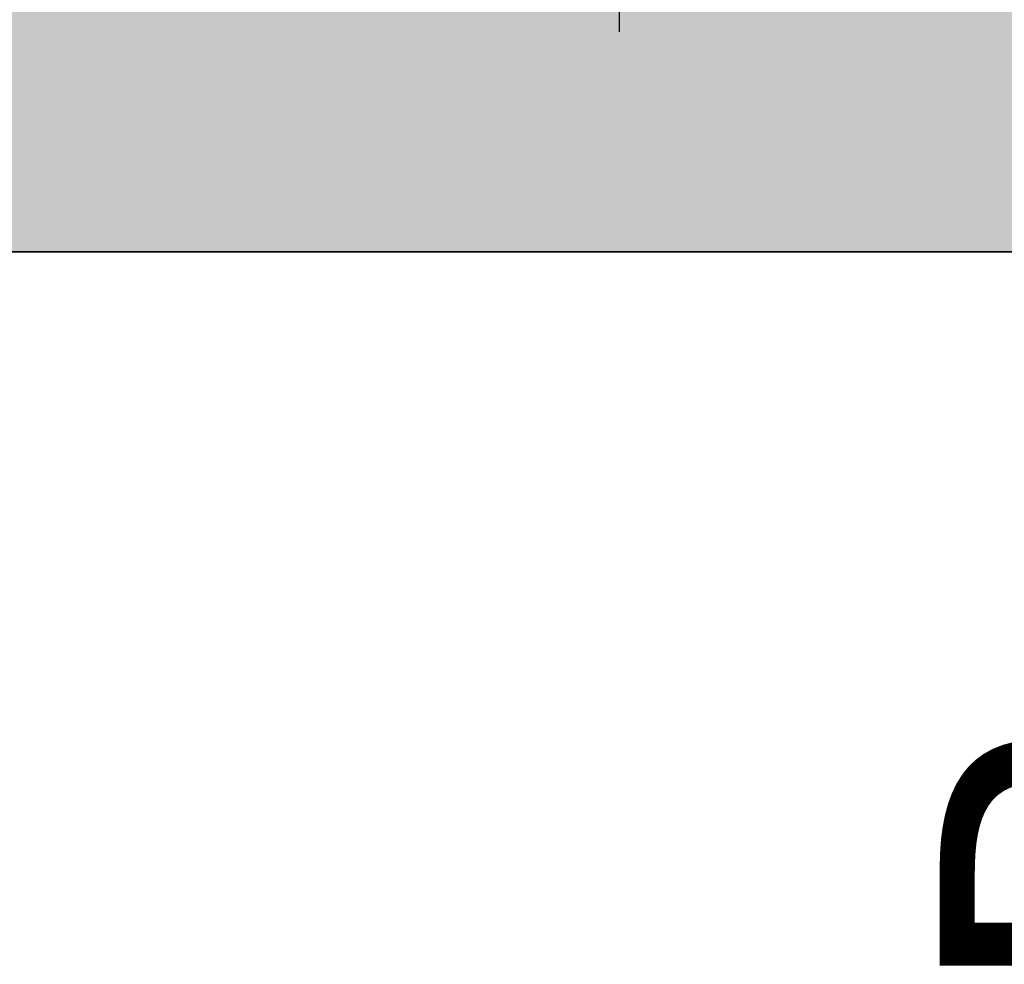
# Model space of a CAD drawing. Units: inches. Extents: x 2083 to 3317, y 1141 to 2115.
# Tile 123 of 256: x 3068 to 3102, y 1238 to 1271. Entities that reach past the tile are written whole.
import ezdxf

# ---------------------------------------------------------------- set-up
doc = ezdxf.new("R2010")
doc.units = ezdxf.units.IN
doc.layers.add('A-ANNO-DIMS', color=2, linetype='Continuous', lineweight=18)
doc.layers.add('A-WALL', color=7, linetype='Continuous', lineweight=35)
doc.layers.add('A-WALL-PATT', color=251, linetype='Continuous', lineweight=13, true_color=0x636466)
doc.styles.get("Standard").update_dxf_attribs({"font": 'arial.ttf'})
doc.dimstyles.new('ISO-25', dxfattribs={"dimtxt": 12, "dimasz": 12, "dimexe": 1.25, "dimexo": 0.625, "dimtad": 1, "dimlunit": 3, "dimtxsty": 'Standard', "dimcen": 2.5, "dimadec": 0, "dimazin": 0, "dimtfac": 1, "dimtmove": 0, "dimatfit": 3, "dimfxl": 1, "dimarcsym": 0})

# ---------------------------------------------------------------- blocks, each defined once
blk = doc.blocks.new('*D10')
at = {"layer": 'A-ANNO-DIMS', "color": 0, "lineweight": -2, "transparency": 16777216}
for p, q in [((2862.96, 1262.636), (2862.96, 1201.384)), ((3126.96, 1262.636), (3126.96, 1201.384)), ((2874.96, 1202.634), (3114.96, 1202.634))]:
    blk.add_line(p, q, dxfattribs=at)
at = {"layer": 'A-ANNO-DIMS', "color": 0, "transparency": 16777216}
for points in [[(2874.96, 1204.634), (2874.96, 1200.634), (2862.96, 1202.634)], [(3114.96, 1204.634), (3114.96, 1200.634), (3126.96, 1202.634)]]:
    blk.add_solid(points, dxfattribs=at)
at = {"layer": 'Defpoints', "color": 0, "transparency": 16777216}
for p in [(2862.96, 1263.261), (3126.96, 1263.261), (3126.96, 1202.634)]:
    blk.add_point(p, dxfattribs=at)
at = {"layer": 'A-ANNO-DIMS', "color": 0, "transparency": 16777216, "insert": (2994.96, 1209.284), "char_height": 12, "attachment_point": 5}
blk.add_mtext("22'", dxfattribs=at)
blk = doc.blocks.new('*D26')
at = {"layer": 'A-ANNO-DIMS', "color": 0, "lineweight": -2, "transparency": 16777216}
for p, q in [((3088.986, 1274.915), (3088.986, 1270.952)), ((3111.24, 1274.915), (3111.24, 1270.952)), ((3076.986, 1272.202), (2840.262, 1272.202)), ((3111.24, 1272.202), (3088.986, 1272.202)), ((3123.24, 1272.202), (3135.24, 1272.202))]:
    blk.add_line(p, q, dxfattribs=at)
at = {"layer": 'A-ANNO-DIMS', "color": 0, "transparency": 16777216}
for points in [[(3076.986, 1274.202), (3076.986, 1270.202), (3088.986, 1272.202)], [(3123.24, 1274.202), (3123.24, 1270.202), (3111.24, 1272.202)]]:
    blk.add_solid(points, dxfattribs=at)
at = {"layer": 'Defpoints', "color": 0, "transparency": 16777216}
for p in [(3088.986, 1275.54), (3111.24, 1275.54), (3088.986, 1272.202)]:
    blk.add_point(p, dxfattribs=at)
at = {"layer": 'A-ANNO-DIMS', "color": 0, "transparency": 16777216, "insert": (2952.624, 1279.032), "char_height": 12, "attachment_point": 5}
blk.add_mtext('NIGHTSTAND 1\'-10 1/2" TYP.', dxfattribs=at)
blk = doc.blocks.new('*D27')
at = {"layer": 'A-ANNO-DIMS', "color": 0, "lineweight": -2, "transparency": 16777216}
for p, q in [((3114.578, 1309.794), (3114.578, 1321.794)), ((3111.865, 1297.794), (3115.828, 1297.794)), ((3114.578, 1297.794), (3114.578, 1275.54)), ((3111.865, 1275.54), (3115.828, 1275.54)), ((3114.578, 1263.54), (3114.578, 1140.989))]:
    blk.add_line(p, q, dxfattribs=at)
at = {"layer": 'A-ANNO-DIMS', "color": 0, "transparency": 16777216}
for points in [[(3112.578, 1309.794), (3116.578, 1309.794), (3114.578, 1297.794)], [(3112.578, 1263.54), (3116.578, 1263.54), (3114.578, 1275.54)]]:
    blk.add_solid(points, dxfattribs=at)
at = {"layer": 'Defpoints', "color": 0, "transparency": 16777216}
for p in [(3111.24, 1297.794), (3111.24, 1275.54), (3114.578, 1275.54)]:
    blk.add_point(p, dxfattribs=at)
at = {"layer": 'A-ANNO-DIMS', "color": 0, "transparency": 16777216, "insert": (3107.749, 1196.264), "char_height": 12, "attachment_point": 5, "rotation": 90}
blk.add_mtext('1\'-10 1/2" TYP.', dxfattribs=at)
blk = doc.blocks.new('*D34')
at = {"layer": 'A-ANNO-DIMS', "color": 0, "lineweight": -2, "transparency": 16777216}
for p, q in [((2226.96, 1262.636), (2226.96, 1209.661)), ((3126.96, 1262.636), (3126.96, 1209.661)), ((2238.96, 1210.911), (3114.96, 1210.911))]:
    blk.add_line(p, q, dxfattribs=at)
at = {"layer": 'A-ANNO-DIMS', "color": 0, "transparency": 16777216}
for points in [[(2238.96, 1212.911), (2238.96, 1208.911), (2226.96, 1210.911)], [(3114.96, 1212.911), (3114.96, 1208.911), (3126.96, 1210.911)]]:
    blk.add_solid(points, dxfattribs=at)
at = {"layer": 'Defpoints', "color": 0, "transparency": 16777216}
for p in [(2226.96, 1263.261), (3126.96, 1263.261), (3126.96, 1210.911)]:
    blk.add_point(p, dxfattribs=at)
at = {"layer": 'A-ANNO-DIMS', "color": 0, "transparency": 16777216, "insert": (2676.96, 1217.663), "char_height": 12, "attachment_point": 5}
blk.add_mtext('75\'-0"', dxfattribs=at)

msp = doc.modelspace()

# ---------------------------------------------------------------- hatches: boundary and pattern name
at = {"layer": 'A-WALL-PATT'}
h = msp.add_hatch(color=256, dxfattribs=at)
h.dxf.hatch_style = 1
h.paths.add_polyline_path([(3126.96, 2020.761), (2748.96, 2020.761), (2604.96, 2020.761), (2226.96, 2020.761), (2226.96, 1702.761), (2466.96, 1702.761), (2466.96, 1582.761), (2418.96, 1582.761), (2418.96, 1477.761), (2226.96, 1477.761), (2226.96, 1263.261), (2544.96, 1263.261), (2544.96, 1411.761), (2604.96, 1411.761), (2685.96, 1411.761), (2685.96, 1420.761), (2604.96, 1420.761), (2604.96, 1573.761), (2604.96, 1702.761), (2604.96, 2011.761), (2748.96, 2011.761), (2748.96, 1702.761), (2862.96, 1702.761), (2862.96, 1621.761), (2871.96, 1621.761), (2871.96, 1702.761), (2883.96, 1702.761), (2883.96, 1706.939, -0.026459), (2883.96, 1711.761), (2757.96, 1711.761), (2757.96, 1807.761), (2787.96, 1807.761), (2787.96, 1812.261), (2757.96, 1812.261), (2757.96, 2011.761), (2877.96, 2011.761), (2877.96, 1812.261), (2847.96, 1812.261), (2847.96, 1807.761), (2889.836, 1807.761), (2889.836, 1812.261), (2882.46, 1812.261), (2882.46, 2011.761), (3117.96, 2011.761), (3117.96, 1812.261), (2937.836, 1812.261), (2937.836, 1807.761), (2995.71, 1807.761), (2995.71, 1796.118), (3000.21, 1796.118), (3000.21, 1807.761), (3117.96, 1807.761), (3117.96, 1711.761), (3000.21, 1711.761), (3000.21, 1760.118), (2998.573, 1760.118, -0.020711), (2995.71, 1760.118), (2995.71, 1711.761), (2931.96, 1711.761), (2931.96, 1702.761), (3126.96, 1702.761)])
h.paths.add_polyline_path([(2471.46, 2011.761), (2471.46, 1810.011), (2462.717, 1810.011), (2462.717, 1805.511), (2505.96, 1805.511), (2505.96, 1810.011), (2475.96, 1810.011), (2475.96, 2011.761), (2595.96, 2011.761), (2595.96, 1810.011), (2565.96, 1810.011), (2565.96, 1805.511), (2595.96, 1805.511), (2595.96, 1711.761), (2235.96, 1711.761), (2235.96, 1805.511), (2353.71, 1805.511), (2353.71, 1796.054), (2358.21, 1796.054), (2358.21, 1805.511), (2414.717, 1805.511), (2414.717, 1810.011), (2235.96, 1810.011), (2235.96, 2011.761)], flags=16)
h.paths.add_polyline_path([(2270.205, 1994.61), (2270.205, 1970.61), (2246.205, 1970.61), (2246.205, 1994.61)], flags=0)
edge = h.paths.add_edge_path(flags=0)
edge.add_ellipse((2332.027, 1899.798), major_axis=(-3.043, 3.043), ratio=0.168252, start_angle=-161.3322, end_angle=-156.3071, ccw=False)
edge.add_ellipse((2333.082, 1898.744), major_axis=(-1.055, 1.055), ratio=0.453532, start_angle=-123.371, end_angle=-94.1591)
edge = h.paths.add_edge_path(flags=0)
edge.add_ellipse((2332.027, 1968.876), major_axis=(3.043, 3.043), ratio=0.168252, start_angle=18.6678, end_angle=23.6929)
edge.add_spline(control_points=[(2332.926, 1970.691), (2332.227, 1970.336), (2330.894, 1969.659), (2328.413, 1970.932), (2327.204, 1967.749), (2324.71, 1969.956), (2322.533, 1967.012), (2320.013, 1971.296), (2317.68, 1968.158), (2316.041, 1967.102), (2315.427, 1966.81)], knot_values=[0, 0, 0, 0, 2.267059, 4.324559, 6.685584, 8.878641, 11.121502, 14.300359, 17.755284, 19.732645, 19.732645, 19.732645, 19.732645], degree=3, periodic=0)
edge.add_ellipse((2332.027, 1968.876), major_axis=(3.043, 3.043), ratio=0.168252, start_angle=18.6678, end_angle=23.6929, ccw=False)
edge.add_ellipse((2333.082, 1969.931), major_axis=(1.055, 1.055), ratio=0.453532, start_angle=56.629, end_angle=85.8409, ccw=False)
edge = h.paths.add_edge_path(flags=0)
edge.add_spline(control_points=[(2296.428, 1967.988), (2293.628, 1965.336), (2287.704, 1959.727), (2299.744, 1949.996), (2294.533, 1935.669), (2290.573, 1920.604), (2293.394, 1909.974), (2296.185, 1904.967)], knot_values=[0.099185, 0.099185, 0.099185, 0.099185, 0.345301, 0.619822, 0.982653, 1.386093, 1.810555, 1.810555, 1.810555, 1.810555], degree=3, periodic=0)
edge.add_spline(control_points=[(2296.185, 1904.967), (2297.384, 1902.619), (2298.001, 1901.949), (2298.553, 1901.468)], knot_values=[0.006246, 0.006246, 0.006246, 0.006246, 0.055476, 0.055476, 0.055476, 0.055476], degree=3, periodic=0)
edge.add_spline(control_points=[(2298.553, 1901.468), (2297.259, 1900.923), (2295.225, 1900.232), (2293.06, 1900.614), (2292.101, 1900.788), (2292.09, 1900.791)], knot_values=[0.312835, 0.312835, 0.312835, 0.312835, 0.40178, 0.474987, 0.475903, 0.475903, 0.475903, 0.475903], degree=3, periodic=0)
edge.add_arc((2292.794, 1904.664), 3.937, 215.4209, 259.6982, ccw=False)
edge.add_spline(control_points=[(2289.585, 1902.382), (2289.477, 1902.535), (2289.368, 1902.688), (2289.261, 1902.841)], knot_values=[0.102872, 0.102872, 0.102872, 0.102872, 0.116896, 0.116896, 0.116896, 0.116896], degree=3, periodic=0)
edge.add_spline(control_points=[(2289.261, 1902.841), (2288.687, 1902.55), (2287.64, 1902.02), (2285.881, 1901.874), (2283.853, 1901.504), (2281.72, 1899.711), (2278.467, 1899.493), (2276.157, 1901.883), (2272.259, 1899.804), (2267.778, 1901.843), (2262.244, 1900.184), (2257.415, 1901.782), (2254.318, 1900.726), (2253.178, 1900.337)], knot_values=[0, 0, 0, 0, 1.907977, 3.477176, 5.261074, 7.972851, 11.680248, 13.717921, 16.939592, 22.789562, 27.502503, 33.595215, 37.145618, 37.145618, 37.145618, 37.145618], degree=3, periodic=0)
edge.add_line((2253.178, 1900.337), (2250.244, 1902.841))
edge.add_line((2250.244, 1902.841), (2250.244, 1965.833))
edge.add_line((2250.244, 1965.833), (2253.178, 1968.337))
edge.add_spline(control_points=[(2253.178, 1968.337), (2254.318, 1967.948), (2257.415, 1966.892), (2262.244, 1968.49), (2267.778, 1966.831), (2271.527, 1968.537), (2273.876, 1967.828), (2274.207, 1967.728)], knot_values=[0, 0, 0, 0, 0.09018, 0.244935, 0.364644, 0.513233, 0.537855, 0.537855, 0.537855, 0.537855], degree=3, periodic=0)
edge.add_arc((2274.353, 1963.793), 3.937, 72.0511, 92.1279, ccw=False)
edge.add_arc((2281.297, 1985.23), 18.596, 252.0511, 288.5657)
edge.add_arc((2292.317, 1956.029), 12.646, 71.0268, 113.7782, ccw=False)
edge = h.paths.add_edge_path(flags=0)
edge.add_spline(control_points=[(2274.899, 1951.856), (2275.066, 1951.617), (2275.233, 1951.377), (2275.398, 1951.136)], knot_values=[1.409916, 1.409916, 1.409916, 1.409916, 1.43159, 1.43159, 1.43159, 1.43159], degree=3, periodic=0)
edge.add_spline(control_points=[(2275.398, 1951.136), (2275.792, 1950.562), (2276.179, 1949.984), (2276.546, 1949.397)], knot_values=[1.358238, 1.358238, 1.358238, 1.358238, 1.409916, 1.409916, 1.409916, 1.409916], degree=3, periodic=0)
edge.add_line((2276.546, 1949.397), (2277.437, 1947.862))
edge.add_spline(control_points=[(2277.437, 1947.862), (2276.304, 1945.673), (2274.64, 1942.427), (2274.632, 1938.094), (2272.799, 1930.852), (2274.356, 1943.897), (2275.948, 1947.923), (2276.546, 1949.397)], knot_values=[0.005632, 0.005632, 0.005632, 0.005632, 0.186014, 0.266002, 0.357087, 0.59639, 0.739732, 0.739732, 0.739732, 0.739732], degree=3, periodic=0)
edge.add_spline(control_points=[(2276.546, 1949.397), (2276.179, 1949.984), (2275.792, 1950.562), (2275.398, 1951.136)], knot_values=[1.358238, 1.358238, 1.358238, 1.358238, 1.409916, 1.409916, 1.409916, 1.409916], degree=3, periodic=0)
edge.add_spline(control_points=[(2275.398, 1951.136), (2274.943, 1950.08), (2274.208, 1948.025), (2273.935, 1944.851), (2272.469, 1937.627), (2273.466, 1945.696), (2274.701, 1951.059), (2274.899, 1951.856)], knot_values=[0.104364, 0.104364, 0.104364, 0.104364, 0.189636, 0.269624, 0.36071, 0.600013, 0.644622, 0.644622, 0.644622, 0.644622], degree=3, periodic=0)
h.paths.add_polyline_path([(2269.168, 1963.128, -0.357527), (2268.171, 1960.976, -0.092561), (2268.171, 1939.436, -0.357527), (2269.168, 1937.285, -0.357527), (2267.016, 1938.282, -0.164785), (2254.686, 1938.282, -0.357527), (2252.534, 1937.285, -0.357527), (2253.531, 1939.436, -0.092561), (2253.531, 1960.976, -0.357527), (2252.534, 1963.128, -0.357527), (2254.686, 1962.131, -0.164785), (2267.016, 1962.131, -0.357527)], flags=0)
h.paths.add_polyline_path([(2248.874, 1967.802), (2248.874, 1957.028), (2249.458, 1957.028), (2249.458, 1911.647), (2248.874, 1911.647), (2248.874, 1900.873), (2246.512, 1900.873, 0.197327), (2244.15, 1902.457), (2244.15, 1966.218, 0.197327), (2246.512, 1967.802)], flags=0)
h.paths.add_polyline_path([(2269.168, 1931.389, -0.357527), (2268.171, 1929.238, -0.092561), (2268.171, 1907.698, -0.357527), (2269.168, 1905.547, -0.357527), (2267.016, 1906.544, -0.164785), (2254.686, 1906.544, -0.357527), (2252.534, 1905.547, -0.357527), (2253.531, 1907.698, -0.092561), (2253.531, 1929.238, -0.357527), (2252.534, 1931.389, -0.357527), (2254.686, 1930.392, -0.164785), (2267.016, 1930.392, -0.357527)], flags=0)
edge = h.paths.add_edge_path(flags=0)
edge.add_spline(control_points=[(2276.197, 1906.724), (2276.168, 1909.029), (2276.114, 1913.372), (2270.598, 1924.925), (2273.905, 1919.013), (2275.922, 1916.262), (2275.475, 1912.402), (2277.258, 1910.381), (2276.696, 1908.225), (2276.646, 1906.813), (2276.618, 1906.008)], knot_values=[0, 0, 0, 0, 8.61026, 16.221274, 18.843057, 23.804898, 27.440828, 29.356102, 31.203478, 33.650687, 33.650687, 33.650687, 33.650687], degree=3, periodic=0)
edge.add_spline(control_points=[(2276.618, 1906.008), (2276.623, 1905.624), (2276.498, 1904.629), (2275.442, 1903.855), (2274.937, 1903.08), (2274.859, 1902.841)], knot_values=[0.156488, 0.156488, 0.156488, 0.156488, 0.184398, 0.231376, 0.250598, 0.250598, 0.250598, 0.250598], degree=3, periodic=0)
edge.add_line((2274.859, 1902.841), (2276.506, 1902.841))
edge.add_spline(control_points=[(2276.506, 1902.841), (2276.788, 1903.085), (2277.665, 1904.125), (2278.25, 1904.341), (2277.654, 1908.527), (2278.156, 1906.228), (2278.1, 1905.286), (2278.847, 1904.069), (2277.857, 1903.415), (2277.874, 1902.991), (2277.904, 1902.841)], knot_values=[0.059574, 0.059574, 0.059574, 0.059574, 0.080753, 0.103741, 0.16972, 0.176036, 0.207137, 0.240474, 0.262341, 0.27366, 0.27366, 0.27366, 0.27366], degree=3, periodic=0)
edge.add_line((2277.904, 1902.841), (2280.03, 1902.841))
edge.add_spline(control_points=[(2280.03, 1902.841), (2279.888, 1903.088), (2279.499, 1903.982), (2280.152, 1905.939), (2278.104, 1909.658), (2279.762, 1907.185), (2280.328, 1904.875), (2280.485, 1903.49), (2281.463, 1903.249), (2281.758, 1902.936), (2281.834, 1902.841)], knot_values=[0.013856, 0.013856, 0.013856, 0.013856, 0.034874, 0.088867, 0.107879, 0.126738, 0.158714, 0.193757, 0.217487, 0.226722, 0.226722, 0.226722, 0.226722], degree=3, periodic=0)
edge.add_spline(control_points=[(2281.834, 1902.841), (2281.788, 1902.827), (2281.647, 1902.783), (2281.396, 1902.859), (2281.088, 1902.985), (2280.721, 1903.061), (2280.333, 1903.026), (2280.125, 1902.899), (2280.03, 1902.841)], knot_values=[0, 0, 0, 0, 0.14413, 0.435517, 0.749276, 1.153046, 1.548371, 1.878348, 1.878348, 1.878348, 1.878348], degree=3, periodic=0)
edge.add_line((2280.03, 1902.841), (2277.904, 1902.841))
edge.add_spline(control_points=[(2277.904, 1902.841), (2277.893, 1902.796), (2277.865, 1902.68), (2277.607, 1902.687), (2277.274, 1902.801), (2276.838, 1902.62), (2276.584, 1902.789), (2276.506, 1902.841)], knot_values=[0, 0, 0, 0, 0.127189, 0.326199, 0.628009, 1.24357, 1.515331, 1.515331, 1.515331, 1.515331], degree=3, periodic=0)
edge.add_line((2276.506, 1902.841), (2274.859, 1902.841))
edge.add_spline(control_points=[(2274.859, 1902.841), (2274.814, 1902.899), (2274.725, 1903.013), (2274.493, 1903.119), (2274.244, 1902.961), (2273.937, 1903.185), (2273.614, 1902.983), (2273.408, 1902.883), (2273.322, 1902.841)], knot_values=[0, 0, 0, 0, 0.21843, 0.436957, 0.687977, 0.990379, 1.398396, 1.69185, 1.69185, 1.69185, 1.69185], degree=3, periodic=0)
edge.add_spline(control_points=[(2273.322, 1902.841), (2273.617, 1903.446), (2274.274, 1904.538), (2276.027, 1904.574), (2276.207, 1906.584), (2276.197, 1906.724)], knot_values=[0.012227, 0.012227, 0.012227, 0.012227, 0.059472, 0.106218, 0.134458, 0.134458, 0.134458, 0.134458], degree=3, periodic=0)
h.paths.add_polyline_path([(2270.776, 1897.79), (2270.776, 1873.79), (2246.776, 1873.79), (2246.776, 1897.79)], flags=0)
h.paths.add_polyline_path([(2353.71, 1760.005), (2353.71, 1760.054), (2358.21, 1760.054, -0.033729)], flags=0)
h.paths.add_polyline_path([(2321.819, 1737.529), (2341.995, 1737.529, -0.414214), (2343.203, 1736.321), (2343.203, 1721.021, -0.414214), (2341.995, 1719.813), (2321.819, 1719.813, -0.414214), (2320.611, 1721.021), (2320.611, 1736.321, -0.414214)], flags=0)
h.paths.add_polyline_path([(2324.235, 1736.321), (2339.579, 1736.321, -0.414214), (2341.995, 1733.905), (2341.995, 1725.45, -0.414214), (2339.579, 1723.034), (2333.681, 1723.034), (2333.845, 1722.045, -0.870646), (2335.425, 1721.826, -0.767327), (2333.923, 1721.423), (2331.291, 1721.423, -0.767327), (2329.788, 1721.826, -0.870646), (2331.368, 1722.045), (2331.533, 1723.034), (2324.235, 1723.034, -0.414214), (2321.819, 1725.45), (2321.819, 1733.905, -0.414214)], flags=0)
h.paths.add_polyline_path([(2570.484, 1928.615), (2589.684, 1928.615), (2590.169, 1928.615), (2590.169, 1904.993), (2570.484, 1904.993)], flags=0)
h.paths.add_polyline_path([(2574.447, 1927.264, -1), (2572.829, 1927.264, -1)], flags=0)
h.paths.add_polyline_path([(2573.09, 1926.941), (2573.925, 1927.776), (2574.148, 1927.553), (2573.313, 1926.718)], flags=0)
h.paths.add_polyline_path([(2578.779, 1919.73, -1), (2571.592, 1919.73, -1)], flags=0)
h.paths.add_polyline_path([(2578.385, 1919.73, -1), (2571.985, 1919.73, -1)], flags=0)
h.paths.add_polyline_path([(2331.596, 1729.476, -1), (2333.618, 1729.476, -1)], flags=0)
h.paths.add_polyline_path([(2578.034, 1927.264, -1), (2576.416, 1927.264, -1)], flags=0)
h.paths.add_polyline_path([(2576.689, 1927.531), (2576.912, 1927.754), (2577.747, 1926.919), (2577.524, 1926.696)], flags=0)
h.paths.add_polyline_path([(2578.139, 1909.86, -1), (2572.232, 1909.86, -1)], flags=0)
h.paths.add_polyline_path([(2577.745, 1909.86, -1), (2572.625, 1909.86, -1)], flags=0)
h.paths.add_polyline_path([(2583.798, 1927.264, -1), (2582.179, 1927.264, -1)], flags=0)
h.paths.add_polyline_path([(2582.719, 1927.754), (2583.554, 1926.919), (2583.331, 1926.696), (2582.496, 1927.531)], flags=0)
h.paths.add_polyline_path([(2582.496, 1927.531), (2582.719, 1927.754), (2583.554, 1926.919), (2583.331, 1926.696)], flags=0)
h.paths.add_polyline_path([(2587.739, 1920.53, -1), (2581.832, 1920.53, -1)], flags=0)
h.paths.add_polyline_path([(2587.345, 1920.53, -1), (2582.225, 1920.53, -1)], flags=0)
h.paths.add_polyline_path([(2587.385, 1927.264, -1), (2585.766, 1927.264, -1)], flags=0)
h.paths.add_polyline_path([(2586.082, 1926.98), (2586.917, 1927.815), (2587.14, 1927.593), (2586.305, 1926.758)], flags=0)
h.paths.add_polyline_path([(2588.379, 1910.66, -1), (2581.192, 1910.66, -1)], flags=0)
h.paths.add_polyline_path([(2587.985, 1910.66, -1), (2581.585, 1910.66, -1)], flags=0)
h.paths.add_polyline_path([(2417.168, 1729.478), (2437.344, 1729.478, -0.414214), (2438.552, 1728.27), (2438.552, 1712.969, -0.414214), (2437.344, 1711.761), (2417.168, 1711.761, -0.414214), (2415.96, 1712.969), (2415.96, 1728.27, -0.414214)], flags=0)
h.paths.add_polyline_path([(2419.584, 1728.27), (2434.928, 1728.27, -0.414214), (2437.344, 1725.854), (2437.344, 1717.398, -0.414214), (2434.928, 1714.983), (2429.029, 1714.983), (2429.194, 1713.994, -0.870646), (2430.774, 1713.775, -0.767327), (2429.271, 1713.372), (2426.64, 1713.372, -0.767327), (2425.137, 1713.775, -0.870646), (2426.717, 1713.994), (2426.882, 1714.983), (2419.584, 1714.983, -0.414214), (2417.168, 1717.398), (2417.168, 1725.854, -0.414214)], flags=0)
h.paths.add_polyline_path([(2419.584, 1728.27), (2434.928, 1728.27, -0.414214), (2437.344, 1725.854), (2437.344, 1717.398, -0.414214), (2434.928, 1714.983), (2429.029, 1714.983), (2428.358, 1719.009), (2427.553, 1719.009), (2426.882, 1714.983), (2419.584, 1714.983, -0.414214), (2417.168, 1717.398), (2417.168, 1725.854, -0.414214)], flags=0)
h.paths.add_polyline_path([(2426.944, 1721.425, -1), (2428.967, 1721.425, -1)], flags=0)
h.paths.add_polyline_path([(2475.96, 1702.761), (2595.96, 1702.761), (2595.96, 1582.761), (2475.96, 1582.761)], flags=16)
h.paths.add_polyline_path([(2427.96, 1573.761), (2595.96, 1573.761), (2595.96, 1468.761), (2595.96, 1420.761), (2384.46, 1420.761), (2384.46, 1468.761), (2427.96, 1468.761)], flags=16)
h.paths.add_polyline_path([(2379.96, 1468.761), (2379.96, 1420.761), (2235.96, 1420.761), (2235.96, 1468.761)], flags=16)
h.paths.add_polyline_path([(2317.816, 1466.696), (2337.992, 1466.696, -0.414214), (2339.2, 1465.488), (2339.2, 1450.187, -0.414214), (2337.992, 1448.979), (2317.816, 1448.979, -0.414214), (2316.608, 1450.187), (2316.608, 1465.488, -0.414214)], flags=0)
h.paths.add_polyline_path([(2320.232, 1465.488), (2335.576, 1465.488, -0.414214), (2337.992, 1463.072), (2337.992, 1454.616, -0.414214), (2335.576, 1452.2), (2329.677, 1452.2), (2329.842, 1451.212, -0.870646), (2331.422, 1450.992, -0.767327), (2329.92, 1450.59), (2327.288, 1450.59, -0.767327), (2325.785, 1450.992, -0.870646), (2327.365, 1451.212), (2327.53, 1452.2), (2320.232, 1452.2, -0.414214), (2317.816, 1454.616), (2317.816, 1463.072, -0.414214)], flags=0)
h.paths.add_polyline_path([(2320.232, 1465.488), (2335.576, 1465.488, -0.414214), (2337.992, 1463.072), (2337.992, 1454.616, -0.414214), (2335.576, 1452.2), (2329.677, 1452.2), (2329.006, 1456.227), (2328.201, 1456.227), (2327.53, 1452.2), (2320.232, 1452.2, -0.414214), (2317.816, 1454.616), (2317.816, 1463.072, -0.414214)], flags=0)
h.paths.add_polyline_path([(2327.593, 1458.643, -1), (2329.615, 1458.643, -1)], flags=0)
h.paths.add_polyline_path([(2244.412, 1433.34), (2241.921, 1433.34, -0.414214), (2240.018, 1435.244), (2240.018, 1440.953, -0.414211), (2241.921, 1442.856), (2244.412, 1442.856, -1.976472)], flags=0)
h.paths.add_polyline_path([(2245.357, 1434.398, -0.414214), (2245.357, 1441.799, -2.144098)], flags=0)
h.paths.add_polyline_path([(2535.96, 1416.261), (2535.96, 1272.261), (2235.96, 1272.261), (2235.96, 1416.261)], flags=16)
h.paths.add_polyline_path([(2260.12, 1384.293), (2260.12, 1362.039), (2237.865, 1362.039), (2237.865, 1384.293)], flags=0)
edge = h.paths.add_edge_path(flags=0)
edge.add_line((2318.252, 1362.093), (2318.146, 1362.001))
edge.add_ellipse((2317.445, 1360.431), major_axis=(2.822, 2.822), ratio=0.168252, start_angle=18.6678, end_angle=20.9481, ccw=False)
edge.add_ellipse((2318.423, 1361.409), major_axis=(0.978, 0.978), ratio=0.453532, start_angle=56.629, end_angle=70.2262, ccw=False)
edge = h.paths.add_edge_path(flags=0)
edge.add_line((2319.107, 1295.571), (2319.015, 1295.677))
edge.add_ellipse((2317.445, 1296.378), major_axis=(-2.822, 2.822), ratio=0.168252, start_angle=-161.3322, end_angle=-159.0519, ccw=False)
edge.add_ellipse((2318.423, 1295.4), major_axis=(-0.978, 0.978), ratio=0.453532, start_angle=-123.371, end_angle=-109.7738)
edge = h.paths.add_edge_path(flags=0)
edge.add_spline(control_points=[(2284.21, 1301.17), (2284.581, 1300.445), (2284.891, 1299.892), (2285.16, 1299.461)], knot_values=[0.039066, 0.039066, 0.039066, 0.039066, 0.055476, 0.055476, 0.055476, 0.055476], degree=3, periodic=0)
edge.add_line((2285.16, 1299.461), (2284.21, 1301.17))
edge = h.paths.add_edge_path(flags=0)
edge.add_line((2280.412, 1297.298), (2283.37, 1297.036))
edge.add_line((2283.37, 1297.036), (2286.406, 1297.926))
edge.add_spline(control_points=[(2286.406, 1297.926), (2285.305, 1297.463), (2284.345, 1297.129), (2283.37, 1297.036)], knot_values=[0.394369, 0.394369, 0.394369, 0.394369, 0.475903, 0.475903, 0.475903, 0.475903], degree=3, periodic=0)
edge.add_spline(control_points=[(2283.37, 1297.036), (2283.281, 1297.028), (2282.316, 1296.957), (2281.313, 1297.134), (2280.423, 1297.296), (2280.412, 1297.298)], knot_values=[0.312835, 0.312835, 0.312835, 0.312835, 0.320246, 0.393453, 0.394369, 0.394369, 0.394369, 0.394369], degree=3, periodic=0)
edge = h.paths.add_edge_path(flags=0)
edge.add_line((2284.436, 1359.607), (2280.446, 1355.328))
edge.add_line((2280.446, 1355.328), (2279.58, 1351.018))
edge.add_line((2279.58, 1351.018), (2282.413, 1346.58))
edge.add_spline(control_points=[(2282.413, 1346.58), (2283.153, 1345.589), (2284.253, 1344.029), (2284.801, 1342.387), (2284.935, 1341.806)], knot_values=[1.240098, 1.240098, 1.240098, 1.240098, 1.332892, 1.382712, 1.382712, 1.382712, 1.382712], degree=3, periodic=0)
edge.add_spline(control_points=[(2284.935, 1341.806), (2285.319, 1340.141), (2285.233, 1338.409), (2284.91, 1336.654)], knot_values=[1.097484, 1.097484, 1.097484, 1.097484, 1.240098, 1.240098, 1.240098, 1.240098], degree=3, periodic=0)
edge.add_spline(control_points=[(2284.91, 1336.654), (2284.587, 1334.899), (2284.027, 1333.12), (2283.463, 1331.361)], knot_values=[0.95487, 0.95487, 0.95487, 0.95487, 1.097484, 1.097484, 1.097484, 1.097484], degree=3, periodic=0)
edge.add_line((2283.463, 1331.361), (2281.89, 1326.153))
edge.add_line((2281.89, 1326.153), (2280.756, 1321.056))
edge.add_line((2280.756, 1321.056), (2280.299, 1316.002))
edge.add_line((2280.299, 1316.002), (2280.716, 1310.95))
edge.add_line((2280.716, 1310.95), (2282.028, 1305.972))
edge.add_line((2282.028, 1305.972), (2284.21, 1301.17))
edge.add_spline(control_points=[(2284.21, 1301.17), (2283.341, 1302.73), (2282.612, 1304.336), (2282.028, 1305.972)], knot_values=[0.099185, 0.099185, 0.099185, 0.099185, 0.241799, 0.241799, 0.241799, 0.241799], degree=3, periodic=0)
edge.add_spline(control_points=[(2282.028, 1305.972), (2281.444, 1307.608), (2281.005, 1309.273), (2280.716, 1310.95)], knot_values=[0.241799, 0.241799, 0.241799, 0.241799, 0.384413, 0.384413, 0.384413, 0.384413], degree=3, periodic=0)
edge.add_spline(control_points=[(2280.716, 1310.95), (2280.433, 1312.588), (2280.289, 1314.277), (2280.299, 1315.962), (2280.299, 1316.002)], knot_values=[0.384413, 0.384413, 0.384413, 0.384413, 0.523647, 0.527028, 0.527028, 0.527028, 0.527028], degree=3, periodic=0)
edge.add_spline(control_points=[(2280.299, 1316.002), (2280.312, 1317.687), (2280.478, 1319.368), (2280.756, 1321.056)], knot_values=[0.527028, 0.527028, 0.527028, 0.527028, 0.669642, 0.669642, 0.669642, 0.669642], degree=3, periodic=0)
edge.add_spline(control_points=[(2280.756, 1321.056), (2281.035, 1322.744), (2281.426, 1324.44), (2281.89, 1326.153)], knot_values=[0.669642, 0.669642, 0.669642, 0.669642, 0.812256, 0.812256, 0.812256, 0.812256], degree=3, periodic=0)
edge.add_spline(control_points=[(2281.89, 1326.153), (2282.264, 1327.533), (2282.788, 1329.262), (2283.353, 1331.018), (2283.463, 1331.361)], knot_values=[0.812256, 0.812256, 0.812256, 0.812256, 0.927087, 0.95487, 0.95487, 0.95487, 0.95487], degree=3, periodic=0)
edge.add_line((2283.463, 1331.361), (2284.91, 1336.654))
edge.add_line((2284.91, 1336.654), (2284.935, 1341.806))
edge.add_line((2284.935, 1341.806), (2282.413, 1346.58))
edge.add_spline(control_points=[(2282.413, 1346.58), (2281.275, 1348.104), (2280.078, 1349.57), (2279.58, 1351.018)], knot_values=[1.382712, 1.382712, 1.382712, 1.382712, 1.525326, 1.525326, 1.525326, 1.525326], degree=3, periodic=0)
edge.add_spline(control_points=[(2279.58, 1351.018), (2279.443, 1351.415), (2279.136, 1352.857), (2279.735, 1354.29), (2280.446, 1355.328)], knot_values=[1.525326, 1.525326, 1.525326, 1.525326, 1.564439, 1.667941, 1.667941, 1.667941, 1.667941], degree=3, periodic=0)
edge.add_spline(control_points=[(2280.446, 1355.328), (2281.426, 1356.758), (2282.931, 1358.183), (2284.436, 1359.607)], knot_values=[1.667941, 1.667941, 1.667941, 1.667941, 1.810555, 1.810555, 1.810555, 1.810555], degree=3, periodic=0)
edge.add_arc((2280.623, 1348.518), 11.726, 71.0268, 113.7782)
edge.add_arc((2270.405, 1375.595), 17.244, 252.0511, 288.5657, ccw=False)
edge.add_arc((2263.966, 1355.718), 3.651, 72.0511, 92.1279)
edge.add_arc((2263.966, 1355.718), 3.651, 92.1279, 177.9851)
edge.add_spline(control_points=[(2260.318, 1355.846), (2260.26, 1354.221), (2260.551, 1350.187), (2262.999, 1346.766), (2264.473, 1344.649)], knot_values=[1.43159, 1.43159, 1.43159, 1.43159, 1.564144, 1.770695, 1.770695, 1.770695, 1.770695], degree=3, periodic=0)
edge.add_line((2264.473, 1344.649), (2264.936, 1343.983))
edge.add_spline(control_points=[(2263.801, 1340.248), (2263.843, 1340.514), (2264.067, 1341.756), (2264.513, 1343.002), (2264.935, 1343.981)], knot_values=[0.53657, 0.53657, 0.53657, 0.53657, 0.559349, 0.644622, 0.644622, 0.644622, 0.644622], degree=3, periodic=0)
edge.add_spline(control_points=[(2264.935, 1343.981), (2265.118, 1343.715), (2265.299, 1343.448), (2265.477, 1343.179)], knot_values=[1.384077, 1.384077, 1.384077, 1.384077, 1.409916, 1.409916, 1.409916, 1.409916], degree=3, periodic=0)
edge.add_spline(control_points=[(2265.477, 1343.179), (2265.655, 1342.911), (2265.829, 1342.641), (2265.999, 1342.369)], knot_values=[1.358238, 1.358238, 1.358238, 1.358238, 1.384077, 1.384077, 1.384077, 1.384077], degree=3, periodic=0)
edge.add_line((2265.999, 1342.369), (2266.826, 1340.946))
edge.add_spline(control_points=[(2266.826, 1340.946), (2268.894, 1337.09), (2271.398, 1325.843), (2270.516, 1310.569), (2275.919, 1301.861), (2277.79, 1299.199)], knot_values=[0.116896, 0.116896, 0.116896, 0.116896, 0.472987, 1.050969, 1.313793, 1.313793, 1.313793, 1.313793], degree=3, periodic=0)
edge.add_spline(control_points=[(2277.79, 1299.199), (2277.839, 1299.128), (2277.889, 1299.057), (2277.94, 1298.987)], knot_values=[0.109884, 0.109884, 0.109884, 0.109884, 0.116896, 0.116896, 0.116896, 0.116896], degree=3, periodic=0)
edge.add_line((2277.94, 1298.987), (2277.789, 1299.199))
edge.add_spline(control_points=[(2277.789, 1299.199), (2277.257, 1298.929), (2276.286, 1298.438), (2275.039, 1298.334), (2274.383, 1298.239), (2274.215, 1298.209)], knot_values=[33.12187, 33.12187, 33.12187, 33.12187, 35.029056, 36.598255, 37.144827, 37.144827, 37.144827, 37.144827], degree=3, periodic=0)
edge.add_line((2274.215, 1298.209), (2273.073, 1297.893))
edge.add_spline(control_points=[(2273.073, 1297.893), (2272.323, 1297.58), (2271.039, 1296.511), (2269.248, 1296.226), (2268.423, 1296.375)], knot_values=[26.532584, 26.532584, 26.532584, 26.532584, 29.198919, 31.839101, 31.839101, 31.839101, 31.839101], degree=3, periodic=0)
edge.add_line((2268.423, 1296.375), (2263.879, 1297.458))
edge.add_spline(control_points=[(2263.879, 1297.458), (2263.556, 1297.359), (2261.86, 1296.839), (2260.239, 1297.282), (2258.933, 1297.516)], knot_values=[15.919551, 15.919551, 15.919551, 15.919551, 16.939592, 21.226067, 21.226067, 21.226067, 21.226067], degree=3, periodic=0)
edge.add_line((2258.933, 1297.516), (2254.055, 1297.329))
edge.add_spline(control_points=[(2254.055, 1297.329), (2253.756, 1297.296), (2252.114, 1297.165), (2250.462, 1297.544), (2249.13, 1297.668)], knot_values=[5.306517, 5.306517, 5.306517, 5.306517, 6.276435, 10.613034, 10.613034, 10.613034, 10.613034], degree=3, periodic=0)
edge.add_line((2249.13, 1297.668), (2244.332, 1296.878))
edge.add_line((2244.332, 1296.878), (2241.611, 1299.199))
edge.add_line((2241.611, 1299.199), (2241.611, 1357.609))
edge.add_line((2241.611, 1357.609), (2244.332, 1359.931))
edge.add_line((2244.332, 1359.931), (2252.729, 1359.543))
edge.add_spline(control_points=[(2252.729, 1359.543), (2252.871, 1359.546), (2253.306, 1359.548), (2253.74, 1359.514), (2254.032, 1359.482)], knot_values=[0.233291, 0.233291, 0.233291, 0.233291, 0.244935, 0.268927, 0.268927, 0.268927, 0.268927], degree=3, periodic=0)
edge.add_line((2254.032, 1359.482), (2259.587, 1359.416))
edge.add_spline(control_points=[(2259.587, 1359.416), (2260.677, 1359.629), (2262.073, 1359.897), (2263.524, 1359.459), (2263.83, 1359.366)], knot_values=[0.422516, 0.422516, 0.422516, 0.422516, 0.513233, 0.537855, 0.537855, 0.537855, 0.537855], degree=3, periodic=0)
edge.add_arc((2263.966, 1355.718), 3.651, 72.0511, 92.1279, ccw=False)
edge.add_arc((2270.405, 1375.595), 17.244, 252.0511, 288.5657)
edge.add_arc((2280.623, 1348.518), 11.726, 71.0268, 113.7782, ccw=False)
h.paths.add_polyline_path([(2240.341, 1359.435), (2240.341, 1349.444), (2240.882, 1349.444), (2240.882, 1307.365), (2240.341, 1307.365), (2240.341, 1297.374), (2238.15, 1297.374, 0.197327), (2235.96, 1298.843), (2235.96, 1357.966, 0.197327), (2238.15, 1359.435)], flags=0)
h.paths.add_polyline_path([(2259.158, 1355.101, -0.357527), (2258.233, 1353.106, -0.092561), (2258.233, 1333.133, -0.357527), (2259.158, 1331.138, -0.357527), (2257.163, 1332.062, -0.164785), (2245.729, 1332.062, -0.357527), (2243.735, 1331.138, -0.357527), (2244.659, 1333.133, -0.092561), (2244.659, 1353.106, -0.357527), (2243.735, 1355.101, -0.357527), (2245.729, 1354.176, -0.164785), (2257.163, 1354.176, -0.357527)], flags=0)
edge = h.paths.add_edge_path(flags=0)
edge.add_line((2265.999, 1342.369), (2266.826, 1340.946))
edge.add_line((2266.826, 1340.946), (2265.308, 1337.814))
edge.add_line((2265.308, 1337.814), (2264.358, 1334.653))
edge.add_line((2264.358, 1334.653), (2264.262, 1333.8))
edge.add_spline(control_points=[(2264.262, 1333.8), (2264.208, 1333.187), (2264.162, 1332.366), (2264.007, 1331.414), (2263.969, 1331.202)], knot_values=[0.464444, 0.464444, 0.464444, 0.464444, 0.516691, 0.531608, 0.531608, 0.531608, 0.531608], degree=3, periodic=0)
edge.add_spline(control_points=[(2263.969, 1331.202), (2263.775, 1330.119), (2263.424, 1328.791), (2263.257, 1328.531), (2263.234, 1328.515)], knot_values=[0.372682, 0.372682, 0.372682, 0.372682, 0.44885, 0.464444, 0.464444, 0.464444, 0.464444], degree=3, periodic=0)
edge.add_spline(control_points=[(2263.234, 1328.515), (2263.096, 1328.42), (2263.131, 1329.301), (2263.275, 1330.616)], knot_values=[0.280919, 0.280919, 0.280919, 0.280919, 0.372682, 0.372682, 0.372682, 0.372682], degree=3, periodic=0)
edge.add_spline(control_points=[(2263.275, 1330.616), (2263.419, 1331.93), (2263.672, 1333.677), (2263.97, 1335.315)], knot_values=[0.189157, 0.189157, 0.189157, 0.189157, 0.280919, 0.280919, 0.280919, 0.280919], degree=3, periodic=0)
edge.add_spline(control_points=[(2263.97, 1335.315), (2264.1, 1336.032), (2264.419, 1337.622), (2264.755, 1338.864), (2264.947, 1339.491)], knot_values=[0.097394, 0.097394, 0.097394, 0.097394, 0.137578, 0.189157, 0.189157, 0.189157, 0.189157], degree=3, periodic=0)
edge.add_spline(control_points=[(2264.947, 1339.491), (2265.29, 1340.606), (2265.644, 1341.494), (2265.999, 1342.369)], knot_values=[0.005632, 0.005632, 0.005632, 0.005632, 0.097394, 0.097394, 0.097394, 0.097394], degree=3, periodic=0)
h.paths.add_polyline_path([(2259.158, 1325.671, -0.357527), (2258.233, 1323.676, -0.092561), (2258.233, 1303.703, -0.357527), (2259.158, 1301.708, -0.357527), (2257.163, 1302.633, -0.164785), (2245.729, 1302.633, -0.357527), (2243.735, 1301.708, -0.357527), (2244.659, 1303.703, -0.092561), (2244.659, 1323.676, -0.357527), (2243.735, 1325.671, -0.357527), (2245.729, 1324.747, -0.164785), (2257.163, 1324.747, -0.357527)], flags=0)
edge = h.paths.add_edge_path(flags=0)
edge.add_spline(control_points=[(2261.709, 1317.311), (2261.679, 1317.418), (2261.762, 1317.389), (2262.491, 1316.09), (2262.962, 1315.301)], knot_values=[14.955861, 14.955861, 14.955861, 14.955861, 16.221274, 18.694826, 18.694826, 18.694826, 18.694826], degree=3, periodic=0)
edge.add_spline(control_points=[(2262.962, 1315.301), (2262.99, 1315.254), (2263.702, 1314.067), (2264.349, 1313.127), (2264.73, 1312.164)], knot_values=[18.694826, 18.694826, 18.694826, 18.694826, 18.843057, 22.433791, 22.433791, 22.433791, 22.433791], degree=3, periodic=0)
edge.add_spline(control_points=[(2264.73, 1312.164), (2264.876, 1311.796), (2265.177, 1310.77), (2265.143, 1309.559), (2265.248, 1308.824)], knot_values=[22.433791, 22.433791, 22.433791, 22.433791, 23.804898, 26.172756, 26.172756, 26.172756, 26.172756], degree=3, periodic=0)
edge.add_line((2265.248, 1308.824), (2265.851, 1307.172))
edge.add_spline(control_points=[(2265.851, 1307.172), (2266.065, 1306.822), (2266.384, 1306.332), (2266.424, 1305.781), (2266.42, 1305.611)], knot_values=[28.062562, 28.062562, 28.062562, 28.062562, 29.356102, 29.911721, 29.911721, 29.911721, 29.911721], degree=3, periodic=0)
edge.add_spline(control_points=[(2266.42, 1305.611), (2266.416, 1305.433), (2266.394, 1305.25), (2266.365, 1305.066)], knot_values=[29.911721, 29.911721, 29.911721, 29.911721, 30.497837, 30.497837, 30.497837, 30.497837], degree=3, periodic=0)
edge.add_line((2266.365, 1305.066), (2266.066, 1302.136))
edge.add_spline(control_points=[(2266.066, 1302.136), (2266.071, 1301.78), (2265.998, 1301.2), (2265.663, 1300.759), (2265.509, 1300.586)], knot_values=[0.156488, 0.156488, 0.156488, 0.156488, 0.184398, 0.203543, 0.203543, 0.203543, 0.203543], degree=3, periodic=0)
edge.add_line((2265.509, 1300.586), (2264.435, 1299.199))
edge.add_line((2264.435, 1299.199), (2265.962, 1299.199))
edge.add_line((2265.962, 1299.199), (2267.336, 1301.175))
edge.add_line((2267.336, 1301.175), (2267.312, 1301.986))
edge.add_spline(control_points=[(2267.312, 1301.986), (2267.261, 1302.862), (2267.16, 1303.737), (2267.271, 1303.326)], knot_values=[0.126229, 0.126229, 0.126229, 0.126229, 0.166617, 0.166617, 0.166617, 0.166617], degree=3, periodic=0)
edge.add_spline(control_points=[(2267.271, 1303.326), (2267.28, 1303.294), (2267.31, 1303.175), (2267.373, 1302.884), (2267.406, 1302.683), (2267.418, 1302.601)], knot_values=[0.166617, 0.166617, 0.166617, 0.166617, 0.16972, 0.176036, 0.180765, 0.180765, 0.180765, 0.180765], degree=3, periodic=0)
edge.add_spline(control_points=[(2267.744, 1300.988), (2267.688, 1301.151), (2267.481, 1301.657), (2267.484, 1302.145), (2267.418, 1302.601)], knot_values=[0.180765, 0.180765, 0.180765, 0.180765, 0.193767, 0.220139, 0.220139, 0.220139, 0.220139], degree=3, periodic=0)
edge.add_line((2267.418, 1302.601), (2267.744, 1300.988))
edge.add_spline(control_points=[(2267.744, 1300.988), (2267.832, 1300.732), (2267.932, 1300.31), (2267.555, 1299.975), (2267.429, 1299.829)], knot_values=[0.220139, 0.220139, 0.220139, 0.220139, 0.240474, 0.25489, 0.25489, 0.25489, 0.25489], degree=3, periodic=0)
edge.add_line((2267.429, 1299.829), (2267.258, 1299.199))
edge.add_line((2267.258, 1299.199), (2269.23, 1299.199))
edge.add_spline(control_points=[(2269.23, 1299.199), (2269.099, 1299.429), (2268.843, 1300.016), (2269.012, 1300.916), (2268.947, 1301.661)], knot_values=[0.013856, 0.013856, 0.013856, 0.013856, 0.034874, 0.067073, 0.067073, 0.067073, 0.067073], degree=3, periodic=0)
edge.add_line((2268.947, 1301.661), (2268.432, 1303.603))
edge.add_spline(control_points=[(2268.432, 1303.603), (2268.176, 1304.192), (2267.596, 1305.251), (2268.041, 1304.623), (2268.251, 1304.282)], knot_values=[0.090155, 0.090155, 0.090155, 0.090155, 0.107879, 0.120289, 0.120289, 0.120289, 0.120289], degree=3, periodic=0)
edge.add_spline(control_points=[(2268.251, 1304.282), (2268.361, 1304.105), (2269.058, 1302.918), (2269.383, 1301.59), (2269.521, 1300.776), (2269.575, 1300.556)], knot_values=[0.120289, 0.120289, 0.120289, 0.120289, 0.126738, 0.158714, 0.173506, 0.173506, 0.173506, 0.173506], degree=3, periodic=0)
edge.add_line((2269.575, 1300.556), (2270.686, 1299.421))
edge.add_spline(control_points=[(2270.686, 1299.421), (2270.767, 1299.357), (2270.838, 1299.281), (2270.903, 1299.199)], knot_values=[0.21816, 0.21816, 0.21816, 0.21816, 0.226722, 0.226722, 0.226722, 0.226722], degree=3, periodic=0)
edge.add_line((2270.937, 1299.193), (2270.903, 1299.199))
edge.add_spline(control_points=[(2270.903, 1299.199), (2270.86, 1299.186), (2270.73, 1299.146), (2270.496, 1299.216), (2270.272, 1299.308), (2270.121, 1299.348), (2270.063, 1299.36)], knot_values=[0.939174, 0.939174, 0.939174, 0.939174, 1.083304, 1.374691, 1.68845, 1.878348, 1.878348, 1.878348, 1.878348], degree=3, periodic=0)
edge.add_line((2270.063, 1299.36), (2269.23, 1299.199))
edge.add_line((2269.23, 1299.199), (2267.258, 1299.199))
edge.add_spline(control_points=[(2267.258, 1299.199), (2267.248, 1299.157), (2267.223, 1299.05), (2266.984, 1299.057), (2266.809, 1299.116), (2266.677, 1299.109), (2266.637, 1299.105)], knot_values=[0.757665, 0.757665, 0.757665, 0.757665, 0.884854, 1.083864, 1.385675, 1.515331, 1.515331, 1.515331, 1.515331], degree=3, periodic=0)
edge.add_spline(control_points=[(2266.637, 1299.105), (2266.485, 1299.089), (2266.236, 1299.017), (2266.035, 1299.151), (2265.962, 1299.199)], knot_values=[0, 0, 0, 0, 0.485905, 0.757665, 0.757665, 0.757665, 0.757665], degree=3, periodic=0)
edge.add_line((2265.962, 1299.199), (2264.435, 1299.199))
edge.add_line((2264.435, 1299.199), (2263.858, 1299.367))
edge.add_spline(control_points=[(2263.858, 1299.367), (2263.819, 1299.371), (2263.78, 1299.386), (2263.74, 1299.402)], knot_values=[0.845925, 0.845925, 0.845925, 0.845925, 0.978627, 0.978627, 0.978627, 0.978627], degree=3, periodic=0)
edge.add_line((2263.722, 1299.396), (2263.01, 1299.199))
edge.add_spline(control_points=[(2263.01, 1299.199), (2263.246, 1299.683), (2263.506, 1300.128), (2263.873, 1300.408)], knot_values=[0.012227, 0.012227, 0.012227, 0.012227, 0.052971, 0.052971, 0.052971, 0.052971], degree=3, periodic=0)
edge.add_spline(control_points=[(2263.873, 1300.408), (2263.932, 1300.453), (2264.084, 1300.553), (2264.255, 1300.624), (2264.36, 1300.665)], knot_values=[0.052971, 0.052971, 0.052971, 0.052971, 0.059472, 0.069086, 0.069086, 0.069086, 0.069086], degree=3, periodic=0)
edge.add_line((2264.36, 1300.665), (2265.142, 1301.078))
edge.add_line((2265.142, 1301.078), (2265.676, 1302.8))
edge.add_line((2265.676, 1302.8), (2265.541, 1305.704))
edge.add_line((2265.541, 1305.704), (2264.803, 1309.328))
edge.add_line((2264.803, 1309.328), (2263.041, 1314.092))
edge.add_spline(control_points=[(2263.041, 1314.092), (2262.384, 1315.671), (2261.796, 1316.998), (2261.709, 1317.311)], knot_values=[11.216896, 11.216896, 11.216896, 11.216896, 14.955861, 14.955861, 14.955861, 14.955861], degree=3, periodic=0)
h.paths.add_polyline_path([(2871.96, 1416.261), (2895.91, 1416.261), (2895.91, 1420.761), (2871.96, 1420.761), (2871.96, 1501.761), (2862.96, 1501.761), (2862.96, 1420.761), (2805.96, 1420.761), (2805.96, 1411.761), (2862.96, 1411.761), (2862.96, 1263.261), (3126.96, 1263.261), (3126.96, 1411.761), (3126.96, 1486.761), (2943.96, 1486.761), (2943.96, 1477.761), (2967.86, 1477.761), (2967.86, 1420.761), (2943.91, 1420.761), (2943.91, 1416.261), (3117.96, 1416.261), (3117.96, 1420.761), (2972.36, 1420.761), (2972.36, 1477.761), (3117.96, 1477.761), (3117.96, 1420.761), (3117.96, 1272.261), (2871.96, 1272.261)], flags=0)
h.paths.add_polyline_path([(2457.126, 1485.943), (2527.603, 1485.943), (2527.603, 1537.636), (2457.126, 1537.636)], flags=8)
h.paths.add_polyline_path([(2481.005, 1609.982), (2590.766, 1609.982), (2590.766, 1682.003), (2481.005, 1682.003)], flags=8)
h.paths.add_polyline_path([(2483.085, 1729.127), (2553.562, 1729.127), (2553.562, 1780.82), (2483.085, 1780.82)], flags=8)
h = msp.add_hatch(color=256, dxfattribs=at)
h.dxf.hatch_style = 1
h.paths.add_polyline_path([(3126.96, 1486.761), (2943.96, 1486.761), (2943.96, 1477.761), (2967.86, 1477.761), (2967.86, 1420.761), (2943.91, 1420.761), (2943.91, 1416.261), (3117.96, 1416.261), (3117.96, 1420.761), (2972.36, 1420.761), (2972.36, 1477.761), (3117.96, 1477.761), (3117.96, 1420.761), (3117.96, 1272.261), (2871.96, 1272.261), (2871.96, 1416.261), (2895.91, 1416.261), (2895.91, 1420.761), (2871.96, 1420.761), (2871.96, 1501.761), (2862.96, 1501.761), (2862.96, 1420.761), (2805.96, 1420.761), (2805.96, 1411.761), (2862.96, 1411.761), (2862.96, 1263.261), (3126.96, 1263.261), (3126.96, 1411.761)])

# ---------------------------------------------------------------- linework, layer by layer
at = {"layer": 'A-WALL'}
msp.add_line((2544.96, 1263.261), (3126.96, 1263.261), dxfattribs=at)

# ---------------------------------------------------------------- dimensions: what is measured, and where the dimension line sits
at = {"layer": 'A-ANNO-DIMS'}
for base, p1, p2, angle, text, picture, middle in [((3114.578, 1275.54), (3111.24, 1297.794), (3111.24, 1275.54), 270, '<> TYP.', '*D27', (3107.749, 1196.264)), ((3088.986, 1272.202), (3111.24, 1275.54), (3088.986, 1275.54), 180, 'NIGHTSTAND <> TYP.', '*D26', (2952.624, 1279.032))]:
    dim = msp.add_linear_dim(base=base, p1=p1, p2=p2, angle=angle, text=text, dimstyle='ISO-25', override={"dimdec": 1, "dimlfac": 1, "dimrnd": 0, "dimzin": 1, "dimdsep": 46, "dimlunit": 4, "dimfrac": 2}, dxfattribs=at)
    dim.commit()
    dim.dimension.update_dxf_attribs({"geometry": picture, "text_midpoint": middle})
for base, p1, override, picture, middle in [((3126.96, 1210.911), (2226.96, 1263.261), {"dimdec": 1, "dimlfac": 1, "dimrnd": 0, "dimzin": 1, "dimdsep": 46, "dimlunit": 4, "dimfrac": 2}, '*D34', (2676.96, 1217.663)), ((3126.96, 1202.634), (2862.96, 1263.261), {"dimclrd": 0, "dimclre": 0, "dimclrt": 0}, '*D10', (2994.96, 1209.284))]:
    dim = msp.add_linear_dim(base=base, p1=p1, p2=(3126.96, 1263.261), dimstyle='ISO-25', override=override, dxfattribs=at)
    dim.commit()
    dim.dimension.update_dxf_attribs({"geometry": picture, "text_midpoint": middle})

doc.saveas('drawing.dxf')
